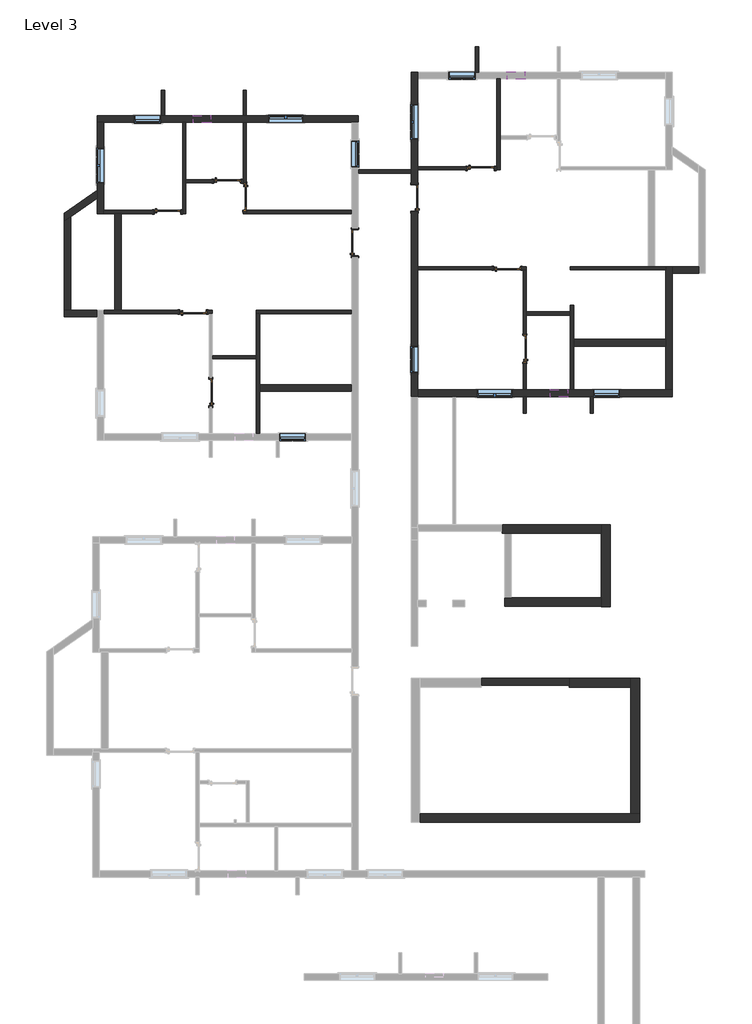
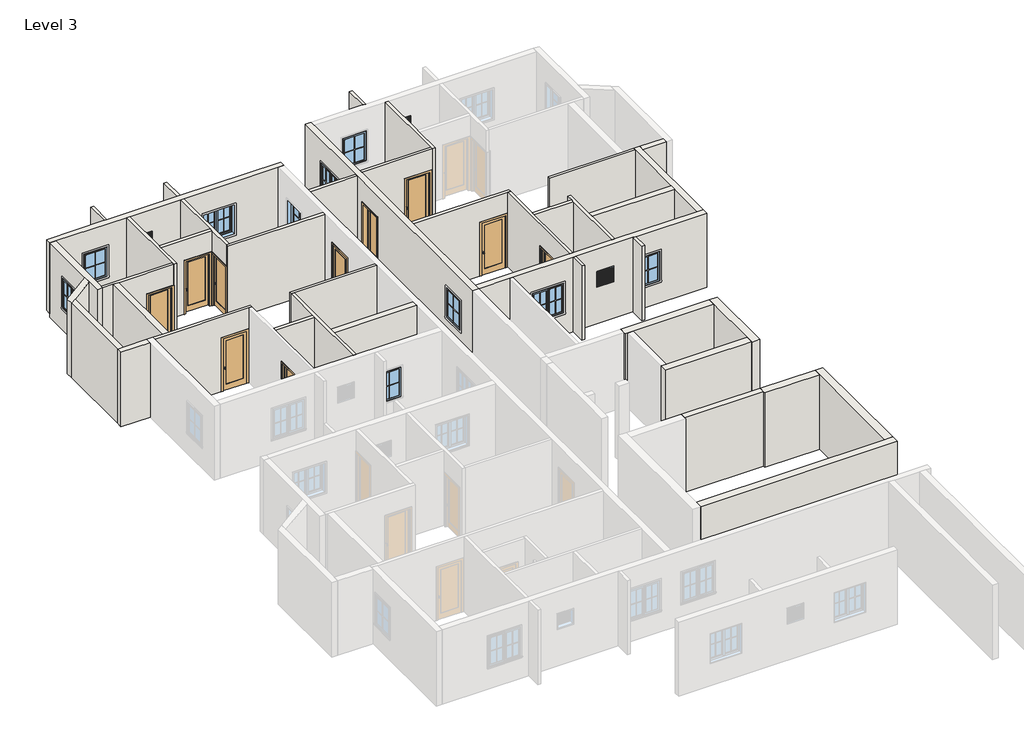
# One storey, part 5 of 7: 41 walls, 13 windows, 10 doors.
"""IFC4 building model written with IfcOpenShell, lengths in millimetres."""

from ifc_helpers import new_model, si_unit, frame, origin, place, context, project, spatial, polyline, outline, extrude, faceted_brep, transform, mapped, element, save
from components import door_3c6ab76a, door_a3feeac7, door_3b97b8e7, door_868ee8a9, window_272f20d6, window_casement_double_4_x_4_af3140d2, window_f2d8fef0

model = new_model("IFC4")

# Units and contexts
model_context = context("Model", 3, world=origin())
ifc_project = project(units=[si_unit("LENGTHUNIT", "METRE", prefix="MILLI")], contexts=[model_context])

# Site, building, storey
site = spatial("IfcSite", under=ifc_project)
building = spatial("IfcBuilding", under=site)
storey = spatial("IfcBuildingStorey", under=building, Name="Level 3", Elevation=3200.4)

# Doors
placement = place(None, origin())
door_shape = door_3c6ab76a(model_context)
element("IfcDoor", 1, ObjectType="Door-Interior-Single-1_Panel-Wood : 2'6\" x 7' door", at=placement, inside=storey, context=model_context, shape_type="MappedRepresentation", body=[
    mapped(door_shape, transform((-10226.9509469, 25492.3711172, 3200.4), x_axis=(1.0, 0.0, 0.0), y_axis=(0.0, 1.0, 0.0), z_axis=(0.0, 0.0, 1.0))),
])
door_2_shape = door_a3feeac7(model_context)
element("IfcDoor", 2, ObjectType="Door-Interior-Single-1_Panel-Wood : 2'6\" x 7' door", at=placement, inside=storey, context=model_context, shape_type="MappedRepresentation", body=[
    mapped(door_2_shape, transform((-10795.2759469, 18161.2961172, 3200.4), x_axis=(0.0, 1.0, 0.0), y_axis=(-1.0, 0.0, 0.0), z_axis=(0.0, 0.0, 1.0))),
])
element("IfcDoor", 3, ObjectType="Door-Interior-Single-1_Panel-Wood : 2'6\" x 7' door", at=placement, inside=storey, context=model_context, shape_type="MappedRepresentation", body=[
    mapped(door_2_shape, transform((101.3240531, 19674.7755084, 3200.4), x_axis=(0.0, 1.0, 0.0), y_axis=(-1.0, 0.0, 0.0), z_axis=(0.0, 0.0, 1.0))),
])
element("IfcDoor", 4, ObjectType="Door-Interior-Single-1_Panel-Wood : 36\" x 84\"", at=placement, inside=storey, context=model_context, shape_type="MappedRepresentation", body=[
    mapped(door_shape, transform((-12297.0509469, 24425.5711172, 3200.4), x_axis=(1.0, 0.0, 0.0), y_axis=(0.0, 1.0, 0.0), z_axis=(0.0, 0.0, 1.0))),
])
element("IfcDoor", 5, ObjectType="Door-Interior-Single-1_Panel-Wood : 36\" x 84\"", at=placement, inside=storey, context=model_context, shape_type="MappedRepresentation", body=[
    mapped(door_shape, transform((-9614.1759469, 24936.7461172, 3200.4), x_axis=(0.0, -1.0, 0.0), y_axis=(1.0, 0.0, 0.0), z_axis=(0.0, 0.0, 1.0))),
])
element("IfcDoor", 6, ObjectType="Door-Interior-Single-1_Panel-Wood : 36\" x 84\"", at=placement, inside=storey, context=model_context, shape_type="MappedRepresentation", body=[
    mapped(door_shape, transform((-1425.8509469, 25939.0505084, 3200.4), x_axis=(1.0, 0.0, 0.0), y_axis=(0.0, 1.0, 0.0), z_axis=(0.0, 0.0, 1.0))),
])
door_3_shape = door_3b97b8e7(model_context)
element("IfcDoor", 7, ObjectType="Door-Interior-Single-1_Panel-Wood : 36\" x 84\"", at=placement, inside=storey, context=model_context, shape_type="MappedRepresentation", body=[
    mapped(door_3_shape, transform((-5791.4759469, 23355.5961172, 3200.4), x_axis=(0.0, 1.0, 0.0), y_axis=(-1.0, 0.0, 0.0), z_axis=(0.0, 0.0, 1.0))),
])
element("IfcDoor", 8, ObjectType="Door-Interior-Single-1_Panel-Wood : 36\" x 84\"", at=placement, inside=storey, context=model_context, shape_type="MappedRepresentation", body=[
    mapped(door_2_shape, transform((-11408.0509469, 20952.1211172, 3200.4), x_axis=(1.0, 0.0, 0.0), y_axis=(0.0, 1.0, 0.0), z_axis=(0.0, 0.0, 1.0))),
])
element("IfcDoor", 9, ObjectType="Door-Interior-Single-1_Panel-Wood : 36\" x 84\"", at=placement, inside=storey, context=model_context, shape_type="MappedRepresentation", body=[
    mapped(door_2_shape, transform((-511.4509469, 22465.6005084, 3200.4), x_axis=(1.0, 0.0, 0.0), y_axis=(0.0, 1.0, 0.0), z_axis=(0.0, 0.0, 1.0))),
])
door_4_shape = door_868ee8a9(model_context)
element("IfcDoor", 10, ObjectType="Door-Interior-Single-1_Panel-Wood : 36\" x 84\"", at=placement, inside=storey, context=model_context, shape_type="MappedRepresentation", body=[
    mapped(door_4_shape, transform((-3727.7259469, 24907.1755084, 3200.4), x_axis=(0.0, 1.0, 0.0), y_axis=(-1.0, 0.0, 0.0), z_axis=(0.0, 0.0, 1.0))),
])

# Walls
element("IfcWall", 11, ObjectType="1' feet", at=placement, inside=storey, context=model_context, shape_type="Brep", body=[
    faceted_brep([(-682.9009469, 13266.6182723, 3200.4), (2758.7990531, 13266.6182723, 3200.4), (2758.7990531, 13266.6182723, 6248.4), (-682.9009469, 13266.6182723, 6248.4), (-682.9009469, 13571.4182723, 3200.4), (-682.9009469, 13571.4182723, 6248.4), (2758.7990531, 13571.4182723, 6248.4), (2758.7990531, 13571.4182723, 3200.4), (-682.9009469, 13342.8182723, 3200.4), (-682.9009469, 13342.8182723, 6248.4)], [[[0, 1, 2, 3]], [[4, 5, 6, 7]], [[1, 0, 8, 4, 7]], [[3, 2, 6, 5, 9]], [[0, 3, 9, 5, 4, 8]], [[2, 1, 7, 6]]]),
])
element("IfcWall", 12, ObjectType="1' feet", at=placement, inside=storey, context=model_context, shape_type="Brep", body=[
    faceted_brep([(3063.5990531, 10726.6182723, 3200.4), (3063.5990531, 13571.4182723, 3200.4), (3063.5990531, 13571.4182723, 6248.4), (3063.5990531, 10726.6182723, 6248.4), (2758.7990531, 10726.6182723, 3200.4), (2758.7990531, 10726.6182723, 6248.4), (2758.7990531, 10739.3182723, 6248.4), (2758.7990531, 11044.1182723, 6248.4), (2758.7990531, 13266.6182723, 6248.4), (2758.7990531, 13571.4182723, 6248.4), (2758.7990531, 13571.4182723, 3200.4), (2758.7990531, 13266.6182723, 3200.4), (2758.7990531, 11044.1182723, 3200.4), (2758.7990531, 10739.3182723, 3200.4)], [[[0, 1, 2, 3]], [[4, 5, 6, 7, 8, 9, 10, 11, 12, 13]], [[1, 0, 4, 13, 12, 11, 10]], [[3, 2, 9, 8, 7, 6, 5]], [[0, 3, 5, 4]], [[2, 1, 10, 9]]]),
])
element("IfcWall", 13, ObjectType="1' feet", at=placement, inside=storey, context=model_context, shape_type="Brep", body=[
    faceted_brep([(2758.7990531, 11044.1182723, 3200.4), (-365.4009469, 11044.1182723, 3200.4), (-594.0009469, 11044.1182723, 3200.4), (-594.0009469, 11044.1182723, 6248.4), (-365.4009469, 11044.1182723, 6248.4), (2758.7990531, 11044.1182723, 6248.4), (2758.7990531, 10739.3182723, 3200.4), (2758.7990531, 10739.3182723, 6248.4), (-594.0009469, 10739.3182723, 6248.4), (-594.0009469, 10739.3182723, 3200.4)], [[[0, 1, 2, 3, 4, 5]], [[6, 7, 8, 9]], [[2, 1, 0, 6, 9]], [[5, 4, 3, 8, 7]], [[0, 5, 7, 6]], [[3, 2, 9, 8]]]),
])
element("IfcWall", 14, ObjectType="1' feet", at=placement, inside=storey, context=model_context, shape_type="Brep", body=[
    faceted_brep([(-3540.4009469, 3245.1461172, 3200.4), (4079.5990531, 3245.1461172, 3200.4), (4079.5990531, 3245.1461172, 6248.4), (-3540.4009469, 3245.1461172, 6248.4), (-3540.4009469, 3549.9461172, 3200.4), (-3540.4009469, 3549.9461172, 6248.4), (3774.7990531, 3549.9461172, 6248.4), (4079.5990531, 3549.9461172, 6248.4), (4079.5990531, 3549.9461172, 3200.4), (3774.7990531, 3549.9461172, 3200.4)], [[[0, 1, 2, 3]], [[4, 5, 6, 7, 8, 9]], [[1, 0, 4, 9, 8]], [[3, 2, 7, 6, 5]], [[2, 1, 8, 7]], [[0, 3, 5, 4]]]),
])
element("IfcWall", 15, ObjectType="1' feet", at=placement, inside=storey, context=model_context, shape_type="Brep", body=[
    faceted_brep([(4079.5990531, 3549.9461172, 3200.4), (4079.5990531, 8236.2461172, 3200.4), (4079.5990531, 8236.2461172, 6248.4), (4079.5990531, 3549.9461172, 6248.4), (3774.7990531, 3549.9461172, 3200.4), (3774.7990531, 3549.9461172, 6248.4), (3774.7990531, 7931.4461172, 6248.4), (3774.7990531, 8236.2461172, 6248.4), (3774.7990531, 8236.2461172, 3200.4), (3774.7990531, 7931.4461172, 3200.4)], [[[0, 1, 2, 3]], [[4, 5, 6, 7, 8, 9]], [[1, 0, 4, 9, 8]], [[3, 2, 7, 6, 5]], [[0, 3, 5, 4]], [[2, 1, 8, 7]]]),
])
element("IfcWall", 16, ObjectType="1' feet", at=placement, inside=storey, context=model_context, shape_type="Brep", body=[
    faceted_brep([(1641.1990531, 7931.4461172, 3200.4), (3774.7990531, 7931.4461172, 3200.4), (3774.7990531, 7931.4461172, 6248.4), (1641.1990531, 7931.4461172, 6248.4), (1641.1990531, 8236.2461172, 3200.4), (1641.1990531, 8236.2461172, 6248.4), (3774.7990531, 8236.2461172, 6248.4), (3774.7990531, 8236.2461172, 3200.4), (1641.1990531, 8007.6461172, 3200.4), (1641.1990531, 8007.6461172, 6248.4)], [[[0, 1, 2, 3]], [[4, 5, 6, 7]], [[1, 0, 8, 4, 7]], [[3, 2, 6, 5, 9]], [[0, 3, 9, 5, 4, 8]], [[2, 1, 7, 6]]]),
])
element("IfcWall", 17, ObjectType="4.5\" wall", at=placement, inside=storey, context=model_context, shape_type="Brep", body=[
    faceted_brep([(-11655.7009469, 24365.2461172, 3200.4), (-11655.7009469, 25432.0461172, 3200.4), (-11655.7009469, 25546.3461172, 3200.4), (-11655.7009469, 27527.5461172, 3200.4), (-11655.7009469, 27527.5461172, 6248.4), (-11655.7009469, 25546.3461172, 6248.4), (-11655.7009469, 25432.0461172, 6248.4), (-11655.7009469, 24365.2461172, 6248.4), (-11770.0009469, 24365.2461172, 3200.4), (-11770.0009469, 24365.2461172, 6248.4), (-11770.0009469, 24479.5461172, 6248.4), (-11770.0009469, 27527.5461172, 6248.4), (-11770.0009469, 27527.5461172, 3200.4), (-11770.0009469, 24479.5461172, 3200.4)], [[[0, 1, 2, 3, 4, 5, 6, 7]], [[8, 9, 10, 11, 12, 13]], [[3, 2, 1, 0, 8, 13, 12]], [[7, 6, 5, 4, 11, 10, 9]], [[4, 3, 12, 11]], [[0, 7, 9, 8]]]),
])
element("IfcWall", 18, ObjectType="4.5\" wall", at=placement, inside=storey, context=model_context, shape_type="SweptSolid", body=[
    extrude(outline(polyline([(6248.4, -9674.5009469), (6248.4, -11655.7009469), (3200.4, -11655.7009469), (3200.4, -10709.5509469), (5359.4, -10709.5509469), (5359.4, -9744.3509469), (3200.4, -9744.3509469), (3200.4, -9674.5009469), (6248.4, -9674.5009469)])), frame((0.0, 25432.0461172, 0.0), z_axis=(0.0, 1.0, 0.0), x_axis=(0.0, 0.0, 1.0)), (0.0, 0.0, 1.0), 114.3),
])
element("IfcWall", 19, ObjectType="4.5\" wall", at=placement, inside=storey, context=model_context, shape_type="Brep", body=[
    faceted_brep([(-11770.0009469, 24365.2461172, 6248.4), (-13903.6009469, 24365.2461172, 6248.4), (-14132.2009469, 24365.2461172, 6248.4), (-14513.2009469, 24365.2461172, 6248.4), (-14513.2009469, 24365.2461172, 3200.4), (-14132.2009469, 24365.2461172, 3200.4), (-13903.6009469, 24365.2461172, 3200.4), (-12779.6509469, 24365.2461172, 3200.4), (-12779.6509469, 24365.2461172, 5359.4), (-11814.4509469, 24365.2461172, 5359.4), (-11814.4509469, 24365.2461172, 3200.4), (-11770.0009469, 24365.2461172, 3200.4), (-14513.2009469, 24479.5461172, 6248.4), (-11770.0009469, 24479.5461172, 6248.4), (-11770.0009469, 24479.5461172, 3200.4), (-11814.4509469, 24479.5461172, 3200.4), (-11814.4509469, 24479.5461172, 5359.4), (-12779.6509469, 24479.5461172, 5359.4), (-12779.6509469, 24479.5461172, 3200.4), (-14513.2009469, 24479.5461172, 3200.4)], [[[0, 1, 2, 3, 4, 5, 6, 7, 8, 9, 10, 11]], [[12, 13, 14, 15, 16, 17, 18, 19]], [[4, 19, 18, 7, 6, 5]], [[14, 11, 10, 15]], [[3, 2, 1, 0, 13, 12]], [[4, 3, 12, 19]], [[0, 11, 14, 13]], [[9, 16, 15, 10]], [[16, 9, 8, 17]], [[17, 8, 7, 18]]]),
])
element("IfcWall", 20, ObjectType="4.5\" wall", at=placement, inside=storey, context=model_context, shape_type="Brep", body=[
    faceted_brep([(-9674.5009469, 24479.5461172, 6248.4), (-9560.2009469, 24479.5461172, 6248.4), (-5902.6009469, 24479.5461172, 6248.4), (-5902.6009469, 24479.5461172, 3200.4), (-9560.2009469, 24479.5461172, 3200.4), (-9560.2009469, 24479.5461172, 5359.4), (-9674.5009469, 24479.5461172, 5359.4), (-9674.5009469, 24365.2461172, 3200.4), (-5902.6009469, 24365.2461172, 3200.4), (-5902.6009469, 24365.2461172, 6248.4), (-9674.5009469, 24365.2461172, 6248.4), (-9674.5009469, 24454.1461172, 3200.4), (-9560.2009469, 24454.1461172, 3200.4), (-9674.5009469, 24454.1461172, 5359.4), (-9560.2009469, 24454.1461172, 5359.4)], [[[0, 1, 2, 3, 4, 5, 6]], [[7, 8, 9, 10]], [[8, 7, 11, 12, 4, 3]], [[2, 1, 0, 10, 9]], [[7, 10, 0, 6, 13, 11]], [[3, 2, 9, 8]], [[12, 14, 5, 4]], [[14, 12, 11, 13]], [[14, 13, 6, 5]]]),
])
element("IfcWall", 21, ObjectType="4.5\" wall", at=placement, inside=storey, context=model_context, shape_type="Brep", body=[
    faceted_brep([(-5902.6009469, 21012.4461172, 3200.4), (-9217.3009469, 21012.4461172, 3200.4), (-9217.3009469, 21012.4461172, 6248.4), (-5902.6009469, 21012.4461172, 6248.4), (-5902.6009469, 20898.1461172, 3200.4), (-5902.6009469, 20898.1461172, 6248.4), (-9103.0009469, 20898.1461172, 6248.4), (-9217.3009469, 20898.1461172, 6248.4), (-9217.3009469, 20898.1461172, 3200.4), (-9103.0009469, 20898.1461172, 3200.4)], [[[0, 1, 2, 3]], [[4, 5, 6, 7, 8, 9]], [[1, 0, 4, 9, 8]], [[3, 2, 7, 6, 5]], [[0, 3, 5, 4]], [[2, 1, 8, 7]]]),
])
element("IfcWall", 22, ObjectType="4.5\" wall", at=placement, inside=storey, context=model_context, shape_type="Brep", body=[
    faceted_brep([(-14513.2009469, 21012.4461172, 6248.4), (-14132.2009469, 21012.4461172, 6248.4), (-13903.6009469, 21012.4461172, 6248.4), (-10741.3009469, 21012.4461172, 6248.4), (-10741.3009469, 21012.4461172, 3200.4), (-10925.4509469, 21012.4461172, 3200.4), (-10925.4509469, 21012.4461172, 5359.4), (-11890.6509469, 21012.4461172, 5359.4), (-11890.6509469, 21012.4461172, 3200.4), (-13903.6009469, 21012.4461172, 3200.4), (-14132.2009469, 21012.4461172, 3200.4), (-14513.2009469, 21012.4461172, 3200.4), (-10741.3009469, 20898.1461172, 6248.4), (-10855.6009469, 20898.1461172, 6248.4), (-14513.2009469, 20898.1461172, 6248.4), (-14513.2009469, 20898.1461172, 3200.4), (-11890.6509469, 20898.1461172, 3200.4), (-11890.6509469, 20898.1461172, 5359.4), (-10925.4509469, 20898.1461172, 5359.4), (-10925.4509469, 20898.1461172, 3200.4), (-10855.6009469, 20898.1461172, 3200.4), (-10741.3009469, 20898.1461172, 3200.4)], [[[0, 1, 2, 3, 4, 5, 6, 7, 8, 9, 10, 11]], [[12, 13, 14, 15, 16, 17, 18, 19, 20, 21]], [[15, 11, 10, 9, 8, 16]], [[4, 21, 20, 19, 5]], [[3, 2, 1, 0, 14, 13, 12]], [[0, 11, 15, 14]], [[4, 3, 12, 21]], [[18, 6, 5, 19]], [[6, 18, 17, 7]], [[7, 17, 16, 8]]]),
])
element("IfcWall", 23, ObjectType="4.5\" wall", at=placement, inside=storey, context=model_context, shape_type="Brep", body=[
    faceted_brep([(-9560.2009469, 27527.5461172, 6248.4), (-9560.2009469, 24479.5461172, 6248.4), (-9560.2009469, 24479.5461172, 5359.4), (-9560.2009469, 25419.3461172, 5359.4), (-9560.2009469, 25419.3461172, 3200.4), (-9560.2009469, 27527.5461172, 3200.4), (-9674.5009469, 24479.5461172, 6248.4), (-9674.5009469, 25432.0461172, 6248.4), (-9674.5009469, 25546.3461172, 6248.4), (-9674.5009469, 27527.5461172, 6248.4), (-9674.5009469, 27527.5461172, 3200.4), (-9674.5009469, 25546.3461172, 3200.4), (-9674.5009469, 25432.0461172, 3200.4), (-9674.5009469, 25419.3461172, 3200.4), (-9674.5009469, 25419.3461172, 5359.4), (-9674.5009469, 24479.5461172, 5359.4)], [[[0, 1, 2, 3, 4, 5]], [[6, 7, 8, 9, 10, 11, 12, 13, 14, 15]], [[10, 5, 4, 13, 12, 11]], [[1, 0, 9, 8, 7, 6]], [[0, 5, 10, 9]], [[1, 6, 15, 2]], [[14, 3, 2, 15]], [[3, 14, 13, 4]]]),
])
element("IfcWall", 24, ObjectType="4.5\" wall", at=placement, inside=storey, context=model_context, shape_type="SweptSolid", body=[
    extrude(outline(polyline([(-9217.3009469, 19323.3461172), (-10741.3009469, 19323.3461172), (-10741.3009469, 19437.6461172), (-9217.3009469, 19437.6461172), (-9217.3009469, 19323.3461172)])), frame((0.0, 0.0, 3200.4), z_axis=(0.0, 0.0, 1.0), x_axis=(1.0, 0.0, 0.0)), (0.0, 0.0, 1.0), 3048.0),
])
element("IfcWall", 25, ObjectType="4.5\" wall", at=placement, inside=storey, context=model_context, shape_type="Brep", body=[
    faceted_brep([(-9217.3009469, 20898.1461172, 3200.4), (-9217.3009469, 19437.6461172, 3200.4), (-9217.3009469, 19323.3461172, 3200.4), (-9217.3009469, 16732.5461172, 3200.4), (-9217.3009469, 16732.5461172, 6248.4), (-9217.3009469, 19323.3461172, 6248.4), (-9217.3009469, 19437.6461172, 6248.4), (-9217.3009469, 20898.1461172, 6248.4), (-9103.0009469, 20898.1461172, 3200.4), (-9103.0009469, 20898.1461172, 6248.4), (-9103.0009469, 18434.3461172, 6248.4), (-9103.0009469, 18205.7461172, 6248.4), (-9103.0009469, 16732.5461172, 6248.4), (-9103.0009469, 16732.5461172, 3200.4), (-9103.0009469, 18205.7461172, 3200.4), (-9103.0009469, 18434.3461172, 3200.4)], [[[0, 1, 2, 3, 4, 5, 6, 7]], [[8, 9, 10, 11, 12, 13, 14, 15]], [[3, 2, 1, 0, 8, 15, 14, 13]], [[7, 6, 5, 4, 12, 11, 10, 9]], [[0, 7, 9, 8]], [[4, 3, 13, 12]]]),
])
element("IfcWall", 26, ObjectType="4.5\" wall", at=placement, inside=storey, context=model_context, shape_type="SweptSolid", body=[
    extrude(outline(polyline([(-5674.0009469, 25878.7255084), (-3845.2009469, 25878.7255084), (-3845.2009469, 25764.4255084), (-5674.0009469, 25764.4255084), (-5674.0009469, 25878.7255084)])), frame((0.0, 0.0, 3200.4), z_axis=(0.0, 0.0, 1.0), x_axis=(1.0, 0.0, 0.0)), (0.0, 0.0, 1.0), 3048.0),
])
element("IfcWall", 27, ObjectType="4.5\" wall", at=placement, inside=storey, context=model_context, shape_type="Brep", body=[
    faceted_brep([(-759.1009469, 25878.7255084, 3200.4), (-759.1009469, 26945.5255084, 3200.4), (-759.1009469, 27059.8255084, 3200.4), (-759.1009469, 29041.0255084, 3200.4), (-759.1009469, 29041.0255084, 6248.4), (-759.1009469, 27059.8255084, 6248.4), (-759.1009469, 26945.5255084, 6248.4), (-759.1009469, 25878.7255084, 6248.4), (-873.4009469, 25878.7255084, 3200.4), (-873.4009469, 25878.7255084, 6248.4), (-873.4009469, 25993.0255084, 6248.4), (-873.4009469, 29041.0255084, 6248.4), (-873.4009469, 29041.0255084, 3200.4), (-873.4009469, 25993.0255084, 3200.4)], [[[0, 1, 2, 3, 4, 5, 6, 7]], [[8, 9, 10, 11, 12, 13]], [[3, 2, 1, 0, 8, 13, 12]], [[7, 6, 5, 4, 11, 10, 9]], [[4, 3, 12, 11]], [[0, 7, 9, 8]]]),
])
element("IfcWall", 28, ObjectType="4.5\" wall", at=placement, inside=storey, context=model_context, shape_type="SweptSolid", body=[
    extrude(outline(polyline([(6248.4, -873.4009469), (6248.4, -3616.6009469), (3200.4, -3616.6009469), (3200.4, -1908.4509469), (5359.4, -1908.4509469), (5359.4, -943.2509469), (3200.4, -943.2509469), (3200.4, -873.4009469), (6248.4, -873.4009469)])), frame((0.0, 25878.7255084, 0.0), z_axis=(0.0, 1.0, 0.0), x_axis=(0.0, 0.0, 1.0)), (0.0, 0.0, 1.0), 114.3),
])
element("IfcWall", 29, ObjectType="4.5\" wall", at=placement, inside=storey, context=model_context, shape_type="Brep", body=[
    faceted_brep([(4993.9990531, 22525.9255084, 3200.4), (4612.9990531, 22525.9255084, 3200.4), (4384.3990531, 22525.9255084, 3200.4), (1679.2990531, 22525.9255084, 3200.4), (1679.2990531, 22525.9255084, 6248.4), (4384.3990531, 22525.9255084, 6248.4), (4612.9990531, 22525.9255084, 6248.4), (4993.9990531, 22525.9255084, 6248.4), (4993.9990531, 22411.6255084, 3200.4), (4993.9990531, 22411.6255084, 6248.4), (1679.2990531, 22411.6255084, 6248.4), (1679.2990531, 22411.6255084, 3200.4)], [[[0, 1, 2, 3, 4, 5, 6, 7]], [[8, 9, 10, 11]], [[3, 2, 1, 0, 8, 11]], [[4, 3, 11, 10]], [[7, 6, 5, 4, 10, 9]], [[0, 7, 9, 8]]]),
])
element("IfcWall", 30, ObjectType="4.5\" wall", at=placement, inside=storey, context=model_context, shape_type="Brep", body=[
    faceted_brep([(155.2990531, 22411.6255084, 6248.4), (40.9990531, 22411.6255084, 6248.4), (-3616.6009469, 22411.6255084, 6248.4), (-3616.6009469, 22411.6255084, 3200.4), (-994.0509469, 22411.6255084, 3200.4), (-994.0509469, 22411.6255084, 5359.4), (-28.8509469, 22411.6255084, 5359.4), (-28.8509469, 22411.6255084, 3200.4), (40.9990531, 22411.6255084, 3200.4), (155.2990531, 22411.6255084, 3200.4), (-3616.6009469, 22525.9255084, 6248.4), (155.2990531, 22525.9255084, 6248.4), (155.2990531, 22525.9255084, 3200.4), (-28.8509469, 22525.9255084, 3200.4), (-28.8509469, 22525.9255084, 5359.4), (-994.0509469, 22525.9255084, 5359.4), (-994.0509469, 22525.9255084, 3200.4), (-3616.6009469, 22525.9255084, 3200.4)], [[[0, 1, 2, 3, 4, 5, 6, 7, 8, 9]], [[10, 11, 12, 13, 14, 15, 16, 17]], [[3, 17, 16, 4]], [[12, 9, 8, 7, 13]], [[2, 1, 0, 11, 10]], [[3, 2, 10, 17]], [[0, 9, 12, 11]], [[6, 14, 13, 7]], [[14, 6, 5, 15]], [[15, 5, 4, 16]]]),
])
element("IfcWall", 31, ObjectType="4.5\" wall", at=placement, inside=storey, context=model_context, shape_type="Brep", body=[
    faceted_brep([(155.2990531, 22411.6255084, 6248.4), (155.2990531, 20951.1255084, 6248.4), (155.2990531, 20836.8255084, 6248.4), (155.2990531, 18246.0255084, 6248.4), (155.2990531, 18246.0255084, 3200.4), (155.2990531, 19192.1755084, 3200.4), (155.2990531, 19192.1755084, 5359.4), (155.2990531, 20157.3755084, 5359.4), (155.2990531, 20157.3755084, 3200.4), (155.2990531, 20836.8255084, 3200.4), (155.2990531, 20951.1255084, 3200.4), (155.2990531, 22411.6255084, 3200.4), (40.9990531, 18246.0255084, 6248.4), (40.9990531, 22411.6255084, 6248.4), (40.9990531, 22411.6255084, 3200.4), (40.9990531, 20157.3755084, 3200.4), (40.9990531, 20157.3755084, 5359.4), (40.9990531, 19192.1755084, 5359.4), (40.9990531, 19192.1755084, 3200.4), (40.9990531, 18246.0255084, 3200.4)], [[[0, 1, 2, 3, 4, 5, 6, 7, 8, 9, 10, 11]], [[12, 13, 14, 15, 16, 17, 18, 19]], [[14, 11, 10, 9, 8, 15]], [[4, 19, 18, 5]], [[3, 2, 1, 0, 13, 12]], [[0, 11, 14, 13]], [[4, 3, 12, 19]], [[7, 16, 15, 8]], [[16, 7, 6, 17]], [[17, 6, 5, 18]]]),
])
element("IfcWall", 32, ObjectType="4.5\" wall", at=placement, inside=storey, context=model_context, shape_type="Brep", body=[
    faceted_brep([(1679.2990531, 21192.4255084, 3200.4), (1679.2990531, 20951.1255084, 3200.4), (1679.2990531, 20836.8255084, 3200.4), (1679.2990531, 18246.0255084, 3200.4), (1679.2990531, 18246.0255084, 6248.4), (1679.2990531, 20836.8255084, 6248.4), (1679.2990531, 20951.1255084, 6248.4), (1679.2990531, 21192.4255084, 6248.4), (1793.5990531, 21192.4255084, 3200.4), (1793.5990531, 21192.4255084, 6248.4), (1793.5990531, 19998.6255084, 6248.4), (1793.5990531, 19770.0255084, 6248.4), (1793.5990531, 18246.0255084, 6248.4), (1793.5990531, 18246.0255084, 3200.4), (1793.5990531, 19770.0255084, 3200.4), (1793.5990531, 19998.6255084, 3200.4)], [[[0, 1, 2, 3, 4, 5, 6, 7]], [[8, 9, 10, 11, 12, 13, 14, 15]], [[3, 2, 1, 0, 8, 15, 14, 13]], [[7, 6, 5, 4, 12, 11, 10, 9]], [[0, 7, 9, 8]], [[4, 3, 13, 12]]]),
])
element("IfcWall", 33, ObjectType="4.5\" wall", at=placement, inside=storey, context=model_context, shape_type="SweptSolid", body=[
    extrude(outline(polyline([(155.2990531, 20951.1255084), (1679.2990531, 20951.1255084), (1679.2990531, 20836.8255084), (155.2990531, 20836.8255084), (155.2990531, 20951.1255084)])), frame((0.0, 0.0, 3200.4), z_axis=(0.0, 0.0, 1.0), x_axis=(1.0, 0.0, 0.0)), (0.0, 0.0, 1.0), 3048.0),
])
element("IfcWall", 34, ObjectType="4.5\" wall", at=placement, inside=storey, context=model_context, shape_type="Brep", body=[
    faceted_brep([(-1617.8862554, 30161.6889788, 3200.4), (-1617.8862554, 29269.6255084, 3200.4), (-1617.8862554, 29269.6255084, 4114.8), (-1617.8862554, 29269.6255084, 5334.0), (-1617.8862554, 29269.6255084, 6248.4), (-1617.8862554, 30161.6889788, 6248.4), (-1503.5862554, 30161.6889788, 3200.4), (-1503.5862554, 30161.6889788, 6248.4), (-1503.5862554, 29269.6255084, 6248.4), (-1503.5862554, 29269.6255084, 3200.4)], [[[0, 1, 2, 3, 4, 5]], [[6, 7, 8, 9]], [[1, 0, 6, 9]], [[5, 4, 8, 7]], [[0, 5, 7, 6]], [[4, 3, 2, 1, 9, 8]]]),
])
element("IfcWall", 35, ObjectType="4.5\" wall", at=placement, inside=storey, context=model_context, shape_type="SweptSolid", body=[
    extrude(outline(polyline([(40.9990531, 17431.8689406), (40.9990531, 18017.4255084), (155.2990531, 18017.4255084), (155.2990531, 17431.8689406), (40.9990531, 17431.8689406)])), frame((0.0, 0.0, 3200.4), z_axis=(0.0, 0.0, 1.0), x_axis=(1.0, 0.0, 0.0)), (0.0, 0.0, 1.0), 3048.0),
])
element("IfcWall", 36, ObjectType="4.5\" wall", at=placement, inside=storey, context=model_context, shape_type="Brep", body=[
    faceted_brep([(2365.0990531, 18017.4255084, 3200.4), (2365.0990531, 17431.8689406, 3200.4), (2365.0990531, 17431.8689406, 6248.4), (2365.0990531, 18017.4255084, 6248.4), (2479.3990531, 18017.4255084, 3200.4), (2479.3990531, 18017.4255084, 4114.8), (2479.3990531, 18017.4255084, 5334.0), (2479.3990531, 18017.4255084, 6248.4), (2479.3990531, 17431.8689406, 6248.4), (2479.3990531, 17431.8689406, 3200.4)], [[[0, 1, 2, 3]], [[4, 5, 6, 7, 8, 9]], [[1, 0, 4, 9]], [[2, 1, 9, 8]], [[3, 2, 8, 7]], [[0, 3, 7, 6, 5, 4]]]),
])
element("IfcWall", 37, ObjectType="4.5\" wall", at=placement, inside=storey, context=model_context, shape_type="SweptSolid", body=[
    extrude(outline(polyline([(-12514.4862554, 27756.1461172), (-12514.4862554, 28648.2095876), (-12400.1862554, 28648.2095876), (-12400.1862554, 27756.1461172), (-12514.4862554, 27756.1461172)])), frame((0.0, 0.0, 3200.4), z_axis=(0.0, 0.0, 1.0), x_axis=(1.0, 0.0, 0.0)), (0.0, 0.0, 1.0), 3048.0),
])
element("IfcWall", 38, ObjectType="4.5\" wall", at=placement, inside=storey, context=model_context, shape_type="SweptSolid", body=[
    extrude(outline(polyline([(-9560.2009469, 28648.2095876), (-9560.2009469, 27756.1461172), (-9674.5009469, 27756.1461172), (-9674.5009469, 28648.2095876), (-9560.2009469, 28648.2095876)])), frame((0.0, 0.0, 3200.4), z_axis=(0.0, 0.0, 1.0), x_axis=(1.0, 0.0, 0.0)), (0.0, 0.0, 1.0), 3048.0),
])
element("IfcWall", 39, ObjectType="9\"", at=placement, inside=storey, context=model_context, shape_type="Brep", body=[
    faceted_brep([(-5674.0009469, 27756.1461172, 3352.8), (-14741.8009469, 27756.1461172, 3352.8), (-14741.8009469, 27756.1461172, 6248.4), (-12514.4862554, 27756.1461172, 6248.4), (-12400.1862554, 27756.1461172, 6248.4), (-9674.5009469, 27756.1461172, 6248.4), (-9560.2009469, 27756.1461172, 6248.4), (-5674.0009469, 27756.1461172, 6248.4), (-10798.4509469, 27756.1461172, 5334.0), (-11408.0509469, 27756.1461172, 5334.0), (-11408.0509469, 27756.1461172, 4724.4), (-10798.4509469, 27756.1461172, 4724.4), (-13447.9362554, 27756.1461172, 5334.0), (-13447.9362554, 27756.1461172, 4114.8), (-12533.5362554, 27756.1461172, 4114.8), (-12533.5362554, 27756.1461172, 5334.0), (-7585.3509469, 27756.1461172, 5334.0), (-8804.5509469, 27756.1461172, 5334.0), (-8804.5509469, 27756.1461172, 4114.8), (-7585.3509469, 27756.1461172, 4114.8), (-5674.0009469, 27527.5461172, 3352.8), (-5674.0009469, 27527.5461172, 6248.4), (-5902.6009469, 27527.5461172, 6248.4), (-9560.2009469, 27527.5461172, 6248.4), (-9674.5009469, 27527.5461172, 6248.4), (-11655.7009469, 27527.5461172, 6248.4), (-11770.0009469, 27527.5461172, 6248.4), (-14513.2009469, 27527.5461172, 6248.4), (-14741.8009469, 27527.5461172, 6248.4), (-14741.8009469, 27527.5461172, 3352.8), (-10798.4509469, 27527.5461172, 5334.0), (-10798.4509469, 27527.5461172, 4724.4), (-11408.0509469, 27527.5461172, 4724.4), (-11408.0509469, 27527.5461172, 5334.0), (-13447.9362554, 27527.5461172, 5334.0), (-12533.5362554, 27527.5461172, 5334.0), (-12533.5362554, 27527.5461172, 4114.8), (-13447.9362554, 27527.5461172, 4114.8), (-7585.3509469, 27527.5461172, 5334.0), (-7585.3509469, 27527.5461172, 4114.8), (-8804.5509469, 27527.5461172, 4114.8), (-8804.5509469, 27527.5461172, 5334.0)], [[[0, 1, 2, 3, 4, 5, 6, 7], [8, 9, 10, 11], [12, 13, 14, 15], [16, 17, 18, 19]], [[20, 21, 22, 23, 24, 25, 26, 27, 28, 29], [30, 31, 32, 33], [34, 35, 36, 37], [38, 39, 40, 41]], [[1, 0, 20, 29]], [[7, 6, 5, 4, 3, 2, 28, 27, 26, 25, 24, 23, 22, 21]], [[2, 1, 29, 28]], [[0, 7, 21, 20]], [[31, 30, 8, 11]], [[32, 31, 11, 10]], [[33, 32, 10, 9]], [[30, 33, 9, 8]], [[13, 12, 34, 37]], [[14, 13, 37, 36]], [[15, 14, 36, 35]], [[12, 15, 35, 34]], [[39, 38, 16, 19]], [[40, 39, 19, 18]], [[41, 40, 18, 17]], [[38, 41, 17, 16]]]),
])
element("IfcWall", 40, ObjectType="9\"", at=placement, inside=storey, context=model_context, shape_type="Brep", body=[
    faceted_brep([(-14741.8009469, 27527.5461172, 3200.4), (-14741.8009469, 25177.6879786, 3200.4), (-14741.8009469, 24898.6461172, 3200.4), (-14741.8009469, 24365.2461172, 3200.4), (-14741.8009469, 24365.2461172, 6248.4), (-14741.8009469, 24898.6461172, 6248.4), (-14741.8009469, 25177.6879786, 6248.4), (-14741.8009469, 27527.5461172, 6248.4), (-14741.8009469, 27527.5461172, 3352.8), (-14741.8009469, 26641.7211172, 5334.0), (-14741.8009469, 25422.5211172, 5334.0), (-14741.8009469, 25422.5211172, 4114.8), (-14741.8009469, 26641.7211172, 4114.8), (-14513.2009469, 27527.5461172, 3200.4), (-14513.2009469, 27527.5461172, 6248.4), (-14513.2009469, 24479.5461172, 6248.4), (-14513.2009469, 24365.2461172, 6248.4), (-14513.2009469, 24365.2461172, 3200.4), (-14513.2009469, 24479.5461172, 3200.4), (-14513.2009469, 26641.7211172, 5334.0), (-14513.2009469, 26641.7211172, 4114.8), (-14513.2009469, 25422.5211172, 4114.8), (-14513.2009469, 25422.5211172, 5334.0)], [[[0, 1, 2, 3, 4, 5, 6, 7, 8], [9, 10, 11, 12]], [[13, 14, 15, 16, 17, 18], [19, 20, 21, 22]], [[3, 2, 1, 0, 13, 18, 17]], [[7, 6, 5, 4, 16, 15, 14]], [[0, 8, 7, 14, 13]], [[4, 3, 17, 16]], [[20, 19, 9, 12]], [[21, 20, 12, 11]], [[22, 21, 11, 10]], [[19, 22, 10, 9]]]),
])
element("IfcWall", 41, ObjectType="9\"", at=placement, inside=storey, context=model_context, shape_type="SweptSolid", body=[
    extrude(outline(polyline([(-13903.6009469, 24365.2461172), (-13903.6009469, 21012.4461172), (-14132.2009469, 21012.4461172), (-14132.2009469, 24365.2461172), (-13903.6009469, 24365.2461172)])), frame((0.0, 0.0, 3200.4), z_axis=(0.0, 0.0, 1.0), x_axis=(1.0, 0.0, 0.0)), (0.0, 0.0, 1.0), 3048.0),
])
element("IfcWall", 42, ObjectType="9\"", at=placement, inside=storey, context=model_context, shape_type="SweptSolid", body=[
    extrude(outline(polyline([(-5902.6009469, 18205.7461172), (-9103.0009469, 18205.7461172), (-9103.0009469, 18434.3461172), (-5902.6009469, 18434.3461172), (-5902.6009469, 18205.7461172)])), frame((0.0, 0.0, 3200.4), z_axis=(0.0, 0.0, 1.0), x_axis=(1.0, 0.0, 0.0)), (0.0, 0.0, 1.0), 3048.0),
])
element("IfcWall", 43, ObjectType="9\"", at=placement, inside=storey, context=model_context, shape_type="Brep", body=[
    faceted_brep([(-3616.6009469, 29269.6255084, 6248.4), (-3616.6009469, 29041.0255084, 6248.4), (-3616.6009469, 25993.0255084, 6248.4), (-3616.6009469, 25878.7255084, 6248.4), (-3616.6009469, 22525.9255084, 6248.4), (-3616.6009469, 22411.6255084, 6248.4), (-3616.6009469, 18246.0255084, 6248.4), (-3616.6009469, 18017.4255084, 6248.4), (-3616.6009469, 18017.4255084, 3200.4), (-3616.6009469, 18246.0255084, 3200.4), (-3616.6009469, 22411.6255084, 3200.4), (-3616.6009469, 22525.9255084, 3200.4), (-3616.6009469, 24424.5755084, 3200.4), (-3616.6009469, 24424.5755084, 5359.4), (-3616.6009469, 25389.7755084, 5359.4), (-3616.6009469, 25389.7755084, 3200.4), (-3616.6009469, 25878.7255084, 3200.4), (-3616.6009469, 25993.0255084, 3200.4), (-3616.6009469, 29041.0255084, 3200.4), (-3616.6009469, 29269.6255084, 3200.4), (-3616.6009469, 19757.3255084, 5334.0), (-3616.6009469, 19757.3255084, 4114.8), (-3616.6009469, 18842.9255084, 4114.8), (-3616.6009469, 18842.9255084, 5334.0), (-3616.6009469, 28155.2005084, 5334.0), (-3616.6009469, 28155.2005084, 4114.8), (-3616.6009469, 26936.0005084, 4114.8), (-3616.6009469, 26936.0005084, 5334.0), (-3845.2009469, 18017.4255084, 6248.4), (-3845.2009469, 25764.4255084, 6248.4), (-3845.2009469, 25878.7255084, 6248.4), (-3845.2009469, 29269.6255084, 6248.4), (-3845.2009469, 29269.6255084, 3200.4), (-3845.2009469, 25878.7255084, 3200.4), (-3845.2009469, 25764.4255084, 3200.4), (-3845.2009469, 25389.7755084, 3200.4), (-3845.2009469, 25389.7755084, 5359.4), (-3845.2009469, 24424.5755084, 5359.4), (-3845.2009469, 24424.5755084, 3200.4), (-3845.2009469, 18017.4255084, 3200.4), (-3845.2009469, 19757.3255084, 5334.0), (-3845.2009469, 18842.9255084, 5334.0), (-3845.2009469, 18842.9255084, 4114.8), (-3845.2009469, 19757.3255084, 4114.8), (-3845.2009469, 28155.2005084, 5334.0), (-3845.2009469, 26936.0005084, 5334.0), (-3845.2009469, 26936.0005084, 4114.8), (-3845.2009469, 28155.2005084, 4114.8)], [[[0, 1, 2, 3, 4, 5, 6, 7, 8, 9, 10, 11, 12, 13, 14, 15, 16, 17, 18, 19], [20, 21, 22, 23], [24, 25, 26, 27]], [[28, 29, 30, 31, 32, 33, 34, 35, 36, 37, 38, 39], [40, 41, 42, 43], [44, 45, 46, 47]], [[32, 19, 18, 17, 16, 15, 35, 34, 33]], [[8, 39, 38, 12, 11, 10, 9]], [[7, 6, 5, 4, 3, 2, 1, 0, 31, 30, 29, 28]], [[0, 19, 32, 31]], [[8, 7, 28, 39]], [[14, 36, 35, 15]], [[36, 14, 13, 37]], [[37, 13, 12, 38]], [[21, 20, 40, 43]], [[22, 21, 43, 42]], [[23, 22, 42, 41]], [[20, 23, 41, 40]], [[25, 24, 44, 47]], [[26, 25, 47, 46]], [[27, 26, 46, 45]], [[24, 27, 45, 44]]]),
])
element("IfcWall", 44, ObjectType="9\"", at=placement, inside=storey, context=model_context, shape_type="Brep", body=[
    faceted_brep([(-3616.6009469, 18017.4255084, 3200.4), (-2402.381873, 18017.4255084, 3200.4), (-2288.081873, 18017.4255084, 3200.4), (40.9990531, 18017.4255084, 3200.4), (155.2990531, 18017.4255084, 3200.4), (2365.0990531, 18017.4255084, 3200.4), (2479.3990531, 18017.4255084, 3200.4), (5222.5990531, 18017.4255084, 3200.4), (5222.5990531, 18017.4255084, 6248.4), (2479.3990531, 18017.4255084, 6248.4), (2365.0990531, 18017.4255084, 6248.4), (155.2990531, 18017.4255084, 6248.4), (40.9990531, 18017.4255084, 6248.4), (-2288.081873, 18017.4255084, 6248.4), (-2402.381873, 18017.4255084, 6248.4), (-3616.6009469, 18017.4255084, 6248.4), (1590.3990531, 18017.4255084, 5334.0), (1590.3990531, 18017.4255084, 4724.4), (980.7990531, 18017.4255084, 4724.4), (980.7990531, 18017.4255084, 5334.0), (2479.3990531, 18017.4255084, 5334.0), (3393.7990531, 18017.4255084, 5334.0), (3393.7990531, 18017.4255084, 4114.8), (2479.3990531, 18017.4255084, 4114.8), (-1552.8509469, 18017.4255084, 5334.0), (-333.6509469, 18017.4255084, 5334.0), (-333.6509469, 18017.4255084, 4114.8), (-1552.8509469, 18017.4255084, 4114.8), (-3616.6009469, 18246.0255084, 3200.4), (-3616.6009469, 18246.0255084, 6248.4), (40.9990531, 18246.0255084, 6248.4), (155.2990531, 18246.0255084, 6248.4), (1679.2990531, 18246.0255084, 6248.4), (1793.5990531, 18246.0255084, 6248.4), (4993.9990531, 18246.0255084, 6248.4), (5222.5990531, 18246.0255084, 6248.4), (5222.5990531, 18246.0255084, 3200.4), (4993.9990531, 18246.0255084, 3200.4), (1793.5990531, 18246.0255084, 3200.4), (1679.2990531, 18246.0255084, 3200.4), (155.2990531, 18246.0255084, 3200.4), (40.9990531, 18246.0255084, 3200.4), (1590.3990531, 18246.0255084, 5334.0), (980.7990531, 18246.0255084, 5334.0), (980.7990531, 18246.0255084, 4724.4), (1590.3990531, 18246.0255084, 4724.4), (2479.3990531, 18246.0255084, 5334.0), (2479.3990531, 18246.0255084, 4114.8), (3393.7990531, 18246.0255084, 4114.8), (3393.7990531, 18246.0255084, 5334.0), (-1552.8509469, 18246.0255084, 5334.0), (-1552.8509469, 18246.0255084, 4114.8), (-333.6509469, 18246.0255084, 4114.8), (-333.6509469, 18246.0255084, 5334.0)], [[[0, 1, 2, 3, 4, 5, 6, 7, 8, 9, 10, 11, 12, 13, 14, 15], [16, 17, 18, 19], [20, 21, 22, 23], [24, 25, 26, 27]], [[28, 29, 30, 31, 32, 33, 34, 35, 36, 37, 38, 39, 40, 41], [42, 43, 44, 45], [46, 47, 48, 49], [50, 51, 52, 53]], [[7, 6, 5, 4, 3, 2, 1, 0, 28, 41, 40, 39, 38, 37, 36]], [[15, 14, 13, 12, 11, 10, 9, 8, 35, 34, 33, 32, 31, 30, 29]], [[0, 15, 29, 28]], [[8, 7, 36, 35]], [[17, 16, 42, 45]], [[18, 17, 45, 44]], [[19, 18, 44, 43]], [[16, 19, 43, 42]], [[47, 46, 20, 23]], [[48, 47, 23, 22]], [[49, 48, 22, 21]], [[46, 49, 21, 20]], [[51, 50, 24, 27]], [[52, 51, 27, 26]], [[53, 52, 26, 25]], [[50, 53, 25, 24]]]),
])
element("IfcWall", 45, ObjectType="9\"", at=placement, inside=storey, context=model_context, shape_type="Brep", body=[
    faceted_brep([(4993.9990531, 22525.9255084, 3200.4), (4993.9990531, 22411.6255084, 3200.4), (4993.9990531, 19998.6255084, 3200.4), (4993.9990531, 19770.0255084, 3200.4), (4993.9990531, 18246.0255084, 3200.4), (4993.9990531, 18246.0255084, 6248.4), (4993.9990531, 19770.0255084, 6248.4), (4993.9990531, 19998.6255084, 6248.4), (4993.9990531, 22411.6255084, 6248.4), (4993.9990531, 22525.9255084, 6248.4), (5222.5990531, 22525.9255084, 3200.4), (5222.5990531, 22525.9255084, 6248.4), (5222.5990531, 22297.3255084, 6248.4), (5222.5990531, 18246.0255084, 6248.4), (5222.5990531, 18246.0255084, 3200.4), (5222.5990531, 22297.3255084, 3200.4)], [[[0, 1, 2, 3, 4, 5, 6, 7, 8, 9]], [[10, 11, 12, 13, 14, 15]], [[4, 3, 2, 1, 0, 10, 15, 14]], [[9, 8, 7, 6, 5, 13, 12, 11]], [[5, 4, 14, 13]], [[0, 9, 11, 10]]]),
])
element("IfcWall", 46, ObjectType="9\"", at=placement, inside=storey, context=model_context, shape_type="SweptSolid", body=[
    extrude(outline(polyline([(4993.9990531, 19770.0255084), (1793.5990531, 19770.0255084), (1793.5990531, 19998.6255084), (4993.9990531, 19998.6255084), (4993.9990531, 19770.0255084)])), frame((0.0, 0.0, 3200.4), z_axis=(0.0, 0.0, 1.0), x_axis=(1.0, 0.0, 0.0)), (0.0, 0.0, 1.0), 3048.0),
])
element("IfcWall", 47, ObjectType="9\"", at=placement, inside=storey, context=model_context, shape_type="SweptSolid", body=[
    extrude(outline(polyline([(1641.1990531, 8007.6461172), (-1406.8009469, 8007.6461172), (-1406.8009469, 8236.2461172), (1641.1990531, 8236.2461172), (1641.1990531, 8007.6461172)])), frame((0.0, 0.0, 3200.4), z_axis=(0.0, 0.0, 1.0), x_axis=(1.0, 0.0, 0.0)), (0.0, 0.0, 1.0), 3048.0),
])
element("IfcWall", 48, ObjectType="9\"", at=placement, inside=storey, context=model_context, shape_type="Brep", body=[
    faceted_brep([(-14741.8009469, 21012.4461172, 3200.4), (-15656.2009469, 21012.4461172, 3200.4), (-15884.8009469, 21012.4461172, 3200.4), (-15884.8009469, 21012.4461172, 6248.4), (-15656.2009469, 21012.4461172, 6248.4), (-14741.8009469, 21012.4461172, 6248.4), (-14741.8009469, 20783.8461172, 3200.4), (-14741.8009469, 20783.8461172, 6248.4), (-15884.8009469, 20783.8461172, 6248.4), (-15884.8009469, 20783.8461172, 3200.4)], [[[0, 1, 2, 3, 4, 5]], [[6, 7, 8, 9]], [[2, 1, 0, 6, 9]], [[5, 4, 3, 8, 7]], [[0, 5, 7, 6]], [[3, 2, 9, 8]]]),
])
element("IfcWall", 49, ObjectType="9\"", at=placement, inside=storey, context=model_context, shape_type="SweptSolid", body=[
    extrude(outline(polyline([(-15656.2009469, 24258.5661172), (-15656.2009469, 21012.4461172), (-15884.8009469, 21012.4461172), (-15884.8009469, 24098.5461172), (-15656.2009469, 24258.5661172)])), frame((0.0, 0.0, 3200.4), z_axis=(0.0, 0.0, 1.0), x_axis=(1.0, 0.0, 0.0)), (0.0, 0.0, 1.0), 3048.0),
])
element("IfcWall", 50, ObjectType="9\"", at=placement, inside=storey, context=model_context, shape_type="Brep", body=[
    faceted_brep([(-15884.8009469, 24098.5461172, 3200.4), (-15656.2009469, 24258.5661172, 3200.4), (-14741.8009469, 24898.6461172, 3200.4), (-14741.8009469, 24898.6461172, 6248.4), (-15656.2009469, 24258.5661172, 6248.4), (-15884.8009469, 24098.5461172, 6248.4), (-15884.8009469, 24377.5879786, 3200.4), (-15884.8009469, 24377.5879786, 6248.4), (-14741.8009469, 25177.6879786, 6248.4), (-14741.8009469, 25177.6879786, 3200.4)], [[[0, 1, 2, 3, 4, 5]], [[6, 7, 8, 9]], [[2, 1, 0, 6, 9]], [[5, 4, 3, 8, 7]], [[3, 2, 9, 8]], [[0, 5, 7, 6]]]),
])
element("IfcWall", 51, ObjectType="9\"", at=placement, inside=storey, context=model_context, shape_type="SweptSolid", body=[
    extrude(outline(polyline([(5222.5990531, 22525.9255084), (6136.9990531, 22525.9255084), (6136.9990531, 22297.3255084), (5222.5990531, 22297.3255084), (5222.5990531, 22525.9255084)])), frame((0.0, 0.0, 3200.4), z_axis=(0.0, 0.0, 1.0), x_axis=(1.0, 0.0, 0.0)), (0.0, 0.0, 1.0), 3048.0),
])

# Windows
window_shape = window_272f20d6(model_context)
element("IfcWindow", 52, ObjectType="Window-Awning-Single : 36\" x 48\"", at=placement, inside=storey, context=model_context, shape_type="MappedRepresentation", body=[
    mapped(window_shape, transform((-12990.7362554, 27641.8461172, 3200.4), x_axis=(-1.0, 0.0, 0.0), y_axis=(0.0, -1.0, 0.0), z_axis=(0.0, 0.0, 1.0))),
])
element("IfcWindow", 53, ObjectType="Window-Awning-Single : 36\" x 48\"", at=placement, inside=storey, context=model_context, shape_type="MappedRepresentation", body=[
    mapped(window_shape, transform((-5788.3009469, 26431.1755084, 3200.4), x_axis=(0.0, -1.0, 0.0), y_axis=(1.0, 0.0, 0.0), z_axis=(0.0, 0.0, 1.0))),
])
element("IfcWindow", 54, ObjectType="Window-Awning-Single : 36\" x 48\"", at=placement, inside=storey, context=model_context, shape_type="MappedRepresentation", body=[
    mapped(window_shape, transform((-7960.0009469, 16618.2461172, 3200.4), x_axis=(-1.0, 0.0, 0.0), y_axis=(0.0, -1.0, 0.0), z_axis=(0.0, 0.0, 1.0))),
])
element("IfcWindow", 55, ObjectType="Window-Awning-Single : 36\" x 48\"", at=placement, inside=storey, context=model_context, shape_type="MappedRepresentation", body=[
    mapped(window_shape, transform((-2075.0862554, 29155.3255084, 3200.4), x_axis=(-1.0, 0.0, 0.0), y_axis=(0.0, -1.0, 0.0), z_axis=(0.0, 0.0, 1.0))),
])
element("IfcWindow", 56, ObjectType="Window-Awning-Single : 36\" x 48\"", at=placement, inside=storey, context=model_context, shape_type="MappedRepresentation", body=[
    mapped(window_shape, transform((2936.5990531, 18131.7255084, 3200.4), x_axis=(-1.0, 0.0, 0.0), y_axis=(0.0, -1.0, 0.0), z_axis=(0.0, 0.0, 1.0))),
])
element("IfcWindow", 57, ObjectType="Window-Awning-Single : 36\" x 48\"", at=placement, inside=storey, context=model_context, shape_type="MappedRepresentation", body=[
    mapped(window_shape, transform((-3730.9009469, 19300.1255084, 3200.4), x_axis=(0.0, 1.0, 0.0), y_axis=(-1.0, 0.0, 0.0), z_axis=(0.0, 0.0, 1.0))),
])
window_casement_double_4_x_4_shape = window_casement_double_4_x_4_af3140d2(model_context)
element("IfcWindow", 58, ObjectType="Window-Casement-Double : 4' x 4'", at=placement, inside=storey, context=model_context, shape_type="MappedRepresentation", body=[
    mapped(window_casement_double_4_x_4_shape, transform((-8194.9509469, 27641.8461172, 3200.4), x_axis=(1.0, 0.0, 0.0), y_axis=(0.0, 1.0, 0.0), z_axis=(0.0, 0.0, 1.0))),
])
element("IfcWindow", 59, ObjectType="Window-Casement-Double : 4' x 4'", at=placement, inside=storey, context=model_context, shape_type="MappedRepresentation", body=[
    mapped(window_casement_double_4_x_4_shape, transform((-14627.5009469, 26032.1211172, 3200.4), x_axis=(0.0, 1.0, 0.0), y_axis=(-1.0, 0.0, 0.0), z_axis=(0.0, 0.0, 1.0))),
])
element("IfcWindow", 60, ObjectType="Window-Casement-Double : 4' x 4'", at=placement, inside=storey, context=model_context, shape_type="MappedRepresentation", body=[
    mapped(window_casement_double_4_x_4_shape, transform((-3730.9009469, 27545.6005084, 3200.4), x_axis=(0.0, 1.0, 0.0), y_axis=(-1.0, 0.0, 0.0), z_axis=(0.0, 0.0, 1.0))),
])
element("IfcWindow", 61, ObjectType="Window-Casement-Double : 4' x 4'", at=placement, inside=storey, context=model_context, shape_type="MappedRepresentation", body=[
    mapped(window_casement_double_4_x_4_shape, transform((-943.2509469, 18131.7255084, 3200.4), x_axis=(-1.0, 0.0, 0.0), y_axis=(0.0, -1.0, 0.0), z_axis=(0.0, 0.0, 1.0))),
])
window_2_shape = window_f2d8fef0(model_context)
element("IfcWindow", 62, ObjectType="Window-Louvers : 24\" x 24\"", at=placement, inside=storey, context=model_context, shape_type="MappedRepresentation", body=[
    mapped(window_2_shape, transform((-11103.2509469, 27635.4961172, 3810.0), x_axis=(-1.0, 0.0, 0.0), y_axis=(0.0, -1.0, 0.0), z_axis=(0.0, 0.0, 1.0))),
])
element("IfcWindow", 63, ObjectType="Window-Louvers : 24\" x 24\"", at=placement, inside=storey, context=model_context, shape_type="MappedRepresentation", body=[
    mapped(window_2_shape, transform((1285.5990531, 18125.3755084, 3810.0), x_axis=(-1.0, 0.0, 0.0), y_axis=(0.0, -1.0, 0.0), z_axis=(0.0, 0.0, 1.0))),
])
element("IfcWindow", 64, ObjectType="Window-Louvers : 24\" x 24\"", at=placement, inside=storey, context=model_context, shape_type="MappedRepresentation", body=[
    mapped(window_2_shape, transform((-213.0009469, 29148.9755084, 3810.0), x_axis=(-1.0, 0.0, 0.0), y_axis=(0.0, -1.0, 0.0), z_axis=(0.0, 0.0, 1.0))),
])

save(model, "model.ifc")

# Revit data of these elements
# Type "Door-Interior-Single-1_Panel-Wood : 2'6\" x 7' door"
#   Type Mark = "9"
#   Assembly Code = "C1020300"
#   Analytic Construction = "Wooden"
#   Top Rail = 0' - 4 11/16"
#   Thickness = 0' - 1 3/8"
#   Thermal Resistance (R) = 2.5876 (h·ft²·°F)/BTU
#   Swing Angle [instance default] = 90.00°
#   Stiles = 0' - 4 3/4"
#   Rough Width = 3' - 2"
#   Rough Height = 7' - 1"
#   Height = 7' - 0"
#   Width = 3' - 0"
#   Heat Transfer Coefficient (U) = 0.3865 BTU/(h·ft²·°F)
#   Bottom Rail = 0' - 9 1/8"
#   Trim Material = Cherry
#   Panel Material = Cherry
#   Frame Material = Cherry
#   Door Handle Material = Aluminum
#   Visual Light Transmittance = 0
#   Solar Heat Gain Coefficient = 0
#   Wall Closure = (empty or 0)
#   Function = (empty or 0)
# Type "Door-Interior-Single-1_Panel-Wood : 36\" x 84\""
#   Type Mark = "8"
#   Assembly Code = "C1020300"
#   Analytic Construction = "Wooden"
#   Top Rail = 0' - 4 11/16"
#   Thickness = 0' - 1 3/8"
#   Thermal Resistance (R) = 2.5876 (h·ft²·°F)/BTU
#   Swing Angle [instance default] = 90.00°
#   Stiles = 0' - 4 3/4"
#   Rough Width = 3' - 2"
#   Rough Height = 7' - 1"
#   Height = 7' - 0"
#   Width = 3' - 0"
#   Heat Transfer Coefficient (U) = 0.3865 BTU/(h·ft²·°F)
#   Bottom Rail = 0' - 9 1/8"
#   Trim Material = Cherry
#   Panel Material = Cherry
#   Frame Material = Cherry
#   Door Handle Material = Aluminum
#   Visual Light Transmittance = 0
#   Solar Heat Gain Coefficient = 0
#   Wall Closure = (empty or 0)
#   Function = (empty or 0)
# Type "1' feet"
#   Assembly Code = "B2010"
#   Layers, outside or top first: 1' - 0" no material (function 1)
# Type "4.5\" wall"
#   Assembly Code = "B2010"
#   Layers, outside or top first: 0' - 4 1/2" no material (function 1)
# Type "9\""
#   Assembly Code = "B2010"
#   Layers, outside or top first: 0' - 9" no material (function 1)
# Type "Window-Awning-Single : 36\" x 48\""
#   Type Mark = "20"
#   Fire Rating = "0.5h"
#   Assembly Code = "B2020100"
#   Analytic Construction = "Double glazing - domestic"
#   Window Inset [instance default] = 0' - 0"
#   Wall Thickness [instance default] = 0' - 6"
#   Visual Light Transmittance = 0.81
#   Thermal Resistance (R) = 1.8146 (h·ft²·°F)/BTU
#   Solar Heat Gain Coefficient = 0.76
#   Rough Width = 3' - 0 1/2"
#   Rough Height = 4' - 0 1/2"
#   Interior Wall Closure [instance default] = 0' - 2 1/4"
#   Height = 4' - 0"
#   Heat Transfer Coefficient (U) = 0.5511 BTU/(h·ft²·°F)
#   Frame Extension [instance default] = 0' - 0 1/4"
#   Exterior Wall Closure [instance default] = 0' - 1 1/4"
#   Extension Jamb [instance default] = 0' - 2 1/4"
#   Default Sill Height = 3' - 0"
#   Width = 3' - 0"
#   Muntin Visibility = yes
#   Interior Trim Visibility [instance default] = yes
#   Exterior Trim Visibility [instance default] = yes
#   Extension Jamb Visibility [instance default] = yes
#   Muntin Pattern = Muntin Pattern_2x2 : Muntin Pattern_2x2
#   Interior Trim Material = Wood - Stained
#   Interior Trim = Trim-Window-Interior-Flat : Picture Frame
#   Interior Frame Material = Wood - Stained
#   Glass Panel Material = Glass
#   Exterior Trim Material = Clad - White
#   Exterior Trim = Trim-Window-Exterior-Flat : with Sill
#   Exterior Frame Material = Clad - White
#   Wall Closure = (empty or 0)
# Type "Window-Casement-Double : 4' x 4'"
#   Type Mark = "21"
#   Fire Rating = "0.5h"
#   Assembly Code = "B2020100"
#   Analytic Construction = "Double glazing - domestic"
#   Frame Extension [instance default] = 0' - 0 1/4"
#   Window Inset [instance default] = 0' - 0"
#   Wall Thickness [instance default] = 0' - 6"
#   Interior Wall Closure [instance default] = 0' - 2 1/4"
#   Half Width = 2' - 0"
#   Visual Light Transmittance = 0.81
#   Thermal Resistance (R) = 1.8146 (h·ft²·°F)/BTU
#   Solar Heat Gain Coefficient = 0.76
#   Rough Width = 4' - 0 1/2"
#   Rough Height = 4' - 0 1/2"
#   Height = 4' - 0"
#   Heat Transfer Coefficient (U) = 0.5511 BTU/(h·ft²·°F)
#   Exterior Wall Closure [instance default] = 0' - 1 1/4"
#   Extension Jamb [instance default] = 0' - 2 1/4"
#   Default Sill Height = 3' - 0"
#   Width = 4' - 0"
#   Muntin Visibility = yes
#   Interior Trim Visibility [instance default] = yes
#   Exterior Trim Visibility [instance default] = yes
#   Extension Jamb Visibility [instance default] = yes
#   Interior Trim Material = Wood - Stained
#   Muntin Pattern = Muntin Pattern_2x2 : Muntin Pattern_2x2
#   Interior Trim = Trim-Window-Interior-Flat : Picture Frame
#   Interior Frame Material = Wood - Stained
#   Glass Panel Material = Glass
#   Exterior Trim Material = Clad - White
#   Exterior Trim = Trim-Window-Exterior-Flat : with Sill
#   Exterior Frame Material = Clad - White
#   Wall Closure = (empty or 0)
# Type "Window-Louvers : 24\" x 24\""
#   Type Mark = "18"
#   Construction Type Id = "GSP4R"
#   Assembly Code = "B20"
#   Analytic Construction = "1/8 in Pilkington single glazing"
#   Visual Light Transmittance = 0.9
#   Thermal Resistance (R) = 1.53941 (h·ft²·°F)/BTU
#   Solar Heat Gain Coefficient = 0.78
#   Max Height = 1' - 11.74264"
#   Height = 2' - 0"
#   Heat Transfer Coefficient (U) = 0.6496 BTU/(h·ft²·°F)
#   Blade Width [instance default] = 1' - 10 1/2"
#   Blade Vertical Thickness = 0' - 0.35355"
#   Blade Thickness = 0' - 0 1/4"
#   Blade Spacing = 0' - 1 1/2"
#   Blade Height = 0' - 1.85355"
#   Blade Depth = 0' - 3"
#   Blade Angle = 45.00°
#   Default Sill Height = 3' - 0"
#   Trim Projection_Exterior = 0' - 0 1/2"
#   Trim Projection_Interior = 0' - 0 1/2"
#   Trim Width_Exterior = 0' - 1 1/2"
#   Trim Width_Interior = 0' - 1 1/2"
#   Width = 2' - 0"
#   Max Blade Count = 12
#   Define Thermal Properties by = 1
#   Blade Count = 12
#   Frame Material = Birch
#   Louver Material = Birch
#   Trim Exterior Material = Birch
#   Trim Interior Material = Birch
#   Wall Closure = (empty or 0)
# Elements 1, 2, 3 (IfcDoor, "Door-Interior-Single-1_Panel-Wood : 2'6\" x 7' door")
#   Swing Angle = 90.00°
#   Phase Created = New Construction
#   Materials on its faces: "Cherry", "Aluminum"
# Elements 4, 5, 6, 7, 8, 9, 10 (IfcDoor, "Door-Interior-Single-1_Panel-Wood : 36\" x 84\"")
#   Swing Angle = 90.00°
#   Phase Created = New Construction
#   Materials on its faces: "Cherry", "Aluminum"
# Elements 11, 12, 13, 14, 15, 16 (IfcWall, "1' feet")
#   Top Offset = 0' - 0"
#   Base Offset = 0' - 0"
#   wall height = 10' - 0"
#   Phase Created = New Construction
#   Base Constraint = Level 3
#   Top Constraint = Level 4
#   Materials on its faces: "Default Wall"
# Elements 17, 18, 19, 20, 21, 22, 23, 24, 25, 26, 27, 28, 29, 30, 31, 32, 33, 34, 35, 36, 37, 38 (IfcWall, "4.5\" wall")
#   Top Offset = 0' - 0"
#   Base Offset = 0' - 0"
#   wall height = 10' - 0"
#   Phase Created = New Construction
#   Base Constraint = Level 3
#   Top Constraint = Level 4
#   Materials on its faces: "Default Wall"
# Element 39 (IfcWall, "9\"")
#   built-in parameter 1001111 = 0' - 6"
#   Top Offset = 10' - 0"
#   Base Offset = 0' - 6"
#   wall height = 9' - 6"
#   Phase Created = New Construction
#   Base Constraint = Level 3
#   Top Constraint = Level 3
#   Materials on its faces: "Default Wall"
# Elements 40, 41, 42, 43, 44, 45, 46, 47, 48, 49, 50, 51 (IfcWall, "9\"")
#   Top Offset = 0' - 0"
#   Base Offset = 0' - 0"
#   wall height = 10' - 0"
#   Phase Created = New Construction
#   Base Constraint = Level 3
#   Top Constraint = Level 4
#   Materials on its faces: "Default Wall"
# Element 52 (IfcWindow, "Window-Awning-Single : 36\" x 48\"")
#   Mark = "18"
#   Window Inset = 0' - 0"
#   Interior Wall Closure = 0' - 2 1/4"
#   Frame Extension = 0' - 0 1/4"
#   Exterior Wall Closure = 0' - 1 1/4"
#   Interior Trim Visibility = yes
#   Exterior Trim Visibility = yes
#   Phase Created = New Construction
#   Materials on its faces: "Wood - Stained", "Glass", "Clad - White"
# Element 53 (IfcWindow, "Window-Awning-Single : 36\" x 48\"")
#   Mark = "19"
#   Window Inset = 0' - 0"
#   Interior Wall Closure = 0' - 2 1/4"
#   Frame Extension = 0' - 0 1/4"
#   Exterior Wall Closure = 0' - 1 1/4"
#   Interior Trim Visibility = yes
#   Exterior Trim Visibility = yes
#   Phase Created = New Construction
#   Materials on its faces: "Wood - Stained", "Glass", "Clad - White"
# Element 54 (IfcWindow, "Window-Awning-Single : 36\" x 48\"")
#   Mark = "20"
#   Window Inset = 0' - 0"
#   Interior Wall Closure = 0' - 2 1/4"
#   Frame Extension = 0' - 0 1/4"
#   Exterior Wall Closure = 0' - 1 1/4"
#   Interior Trim Visibility = yes
#   Exterior Trim Visibility = yes
#   Phase Created = New Construction
#   Materials on its faces: "Wood - Stained", "Glass", "Clad - White"
# Element 55 (IfcWindow, "Window-Awning-Single : 36\" x 48\"")
#   Mark = "22"
#   Window Inset = 0' - 0"
